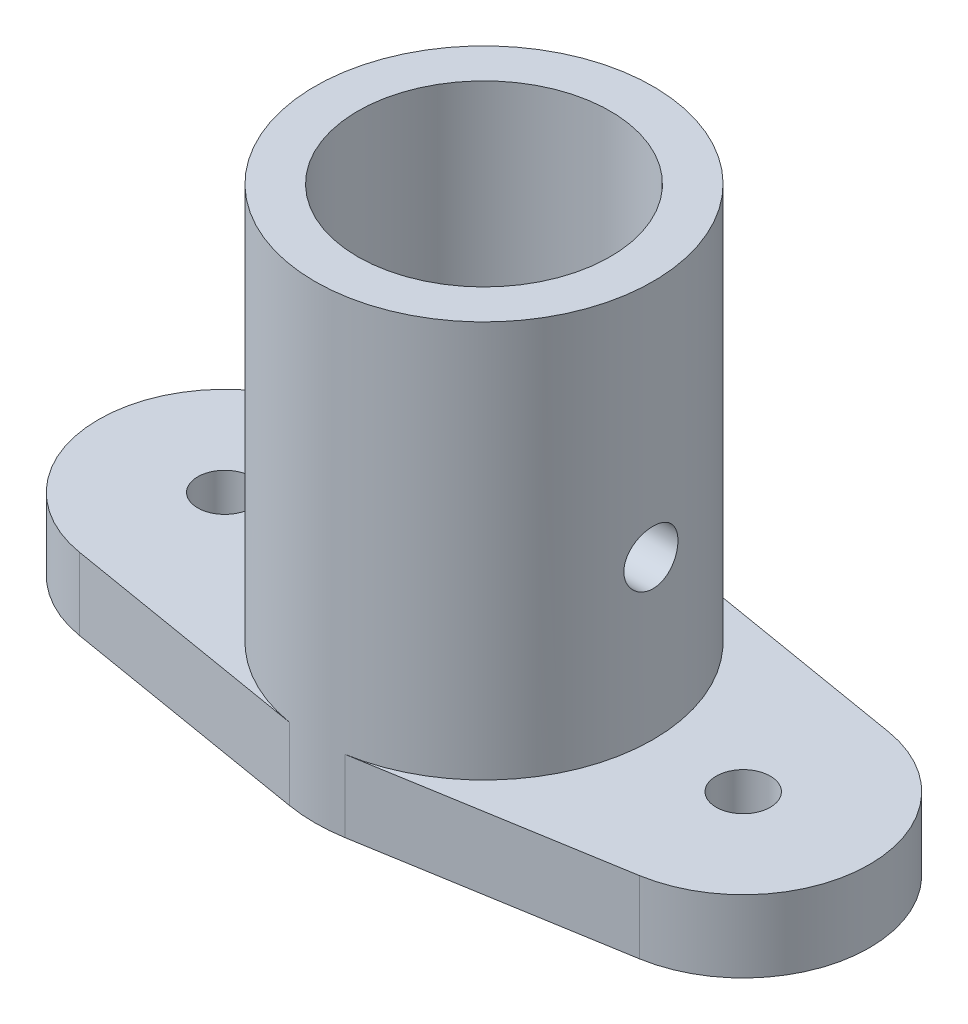
from build123d import *
from build123d.topology import SkipClean

# Parameters (mm, degrees)
BASE_FLANGE_SKETCH_R     = 6
BASE_FLANGE_DEPTH        = 8
TUBE_START               = 88
TUBE_SKETCH_R            = 37.5
TUBE_75_DEPTH            = 88
BORE_SKETCH_R            = 28
BORE_56_DEPTH            = 76
SPIGOT_SKETCH_R          = 19
SPIGOT_38_DEPTH          = 6
SPIGOT_HOLE_SKETCH_R     = 11
SPIGOT_HOLE_22_DEPTH     = 22
BORE_STEP_SKETCH_R       = 22.5
BORE_STEP_45_DEPTH       = 12
CROSS_HOLE_12_DEPTH      = 134.912284724
CROSS_HOLE_12_DEPTH_BACK = 134.912284724
CROSS_HOLE_SKETCH_R      = 6


with BuildPart() as part:
    # Base Flange Sketch → Base Flange (new, symmetric)
    with BuildSketch(Plane(origin=(0, 0, 0), x_dir=(1, 0, 0), z_dir=(0, 1, 0))):
        with BuildLine():
            Line((-62.126086957, -27.615200877), (-6.195652174, -36.984644032))
            ThreePointArc((-6.195652174, -36.984644032), (0, -37.5), (6.195652174, -36.984644032))
            Line((6.195652174, -36.984644032), (62.126086957, -27.615200877))
            ThreePointArc((62.126086957, -27.615200877), (85.5, 0), (62.126086957, 27.615200877))
            Line((62.126086957, 27.615200877), (6.195652174, 36.984644032))
            ThreePointArc((6.195652174, 36.984644032), (0, 37.5), (-6.195652174, 36.984644032))
            Line((-6.195652174, 36.984644032), (-62.126086957, 27.615200877))
            ThreePointArc((-62.126086957, 27.615200877), (-85.5, 0), (-62.126086957, -27.615200877))
        make_face()
        with Locations(Location((-57.5, 0, 0), (0, 0, 270))):
            Circle(BASE_FLANGE_SKETCH_R, mode=Mode.SUBTRACT)
        with Locations(Location((57.5, 0, 0), (0, 0, 270))):
            Circle(BASE_FLANGE_SKETCH_R, mode=Mode.SUBTRACT)
    extrude(amount=BASE_FLANGE_DEPTH, both=True)

    # Tube Sketch → Tube Ø75 (add)
    with SkipClean():  # the faces are left unmerged after this step: merging them gives an invalid solid
        with BuildSketch(Plane(origin=(0, 8, 0), x_dir=(1, 0, 0), z_dir=(0, 1, 0)).offset(TUBE_START)):
            with Locations(Location((0, 0, 0), (0, 0, 99.5098634))):
                Circle(TUBE_SKETCH_R)
        extrude(amount=-TUBE_75_DEPTH)

    # Bore Sketch → Bore Ø56 (cut)
    with SkipClean():  # the faces are left unmerged after this step: merging them gives an invalid solid
        with BuildSketch(Plane(origin=(0, 96, 0), x_dir=(1, 0, 0), z_dir=(0, 1, 0))):
            with Locations(Location((0, 0, 0), (0, 0, 270))):
                Circle(BORE_SKETCH_R)
        extrude(amount=-BORE_56_DEPTH, mode=Mode.SUBTRACT)

    # Spigot Sketch → Spigot Ø38 (add)
    with SkipClean():  # the faces are left unmerged after this step: merging them gives an invalid solid
        with BuildSketch(Plane.XZ.offset(8)):
            with Locations(Location((0, 0, 0), (0, 0, 270))):
                Circle(SPIGOT_SKETCH_R)
        extrude(amount=SPIGOT_38_DEPTH)

    # Spigot Hole Sketch → Spigot Hole Ø22 (cut)
    with SkipClean():  # the faces are left unmerged after this step: merging them gives an invalid solid
        with BuildSketch(Plane.XZ.offset(14)):
            with Locations(Location((0, 0, 0), (0, 0, 270))):
                Circle(SPIGOT_HOLE_SKETCH_R)
        extrude(amount=-SPIGOT_HOLE_22_DEPTH, mode=Mode.SUBTRACT)

    # Bore Step Sketch → Bore Step Ø45 (cut)
    with SkipClean():  # the faces are left unmerged after this step: merging them gives an invalid solid
        with BuildSketch(Plane(origin=(0, 20, 0), x_dir=(1, 0, 0), z_dir=(0, 1, 0))):
            with Locations(Location((0, 0, 0), (0, 0, 270))):
                Circle(BORE_STEP_SKETCH_R)
        extrude(amount=-BORE_STEP_45_DEPTH, mode=Mode.SUBTRACT)

    # Cross Hole Sketch → Cross Hole Ø12 (cut, two sides: drawn at the far end of the back side and taken through both)
    with SkipClean():  # the faces are left unmerged after this step: merging them gives an invalid solid
        with BuildSketch(Plane(origin=(0, 0, 0), x_dir=(0, 0, -1), z_dir=(1, 0, 0)).offset(-CROSS_HOLE_12_DEPTH_BACK)):
            with Locations((0, 43)):
                Circle(CROSS_HOLE_SKETCH_R)
        extrude(amount=CROSS_HOLE_12_DEPTH + CROSS_HOLE_12_DEPTH_BACK, mode=Mode.SUBTRACT)


solid = part.part
